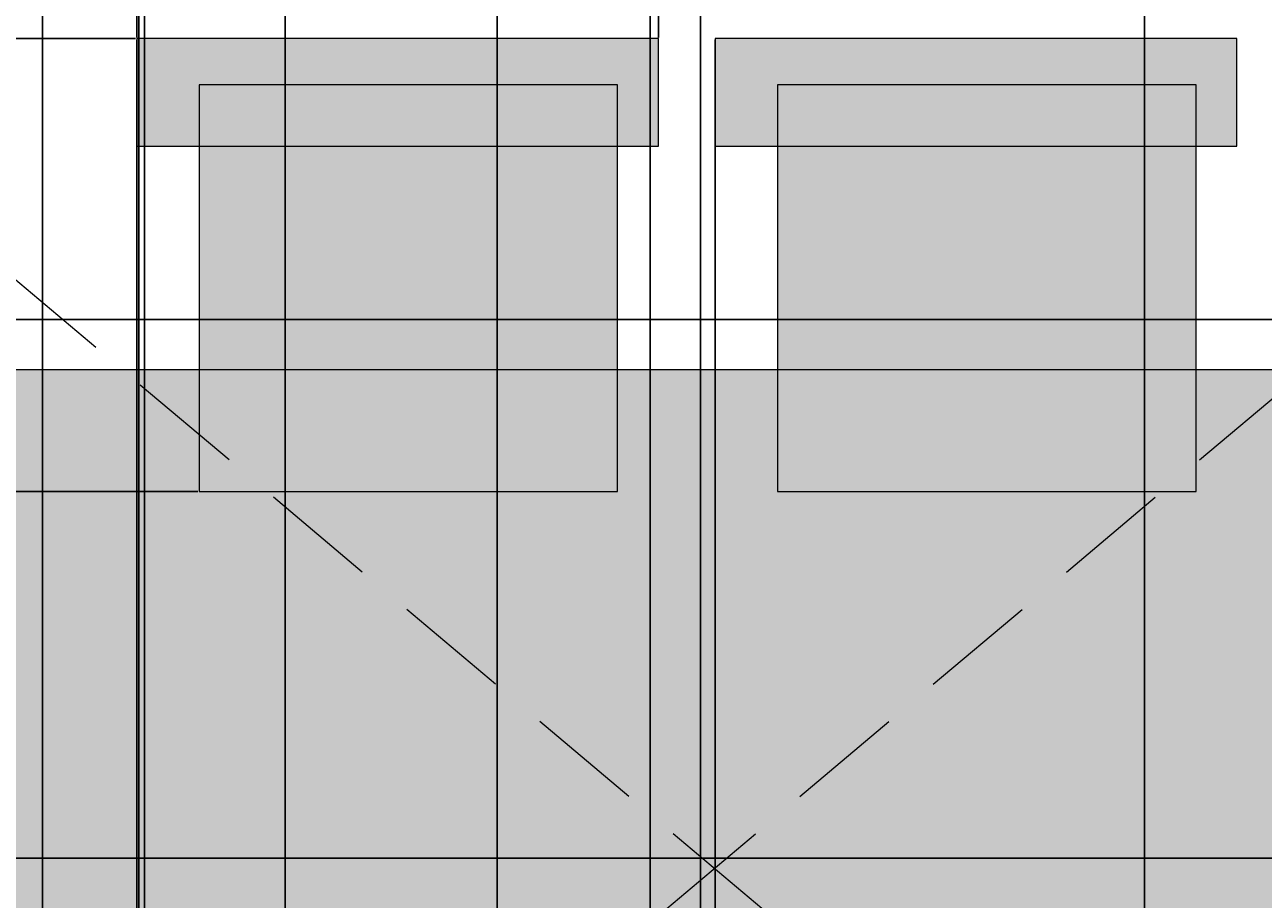
# Model space of a CAD drawing. Units: inches. Extents: x 818 to 1898, y 976 to 2364.
# Tile 73 of 96: x 1305 to 1372, y 1980 to 2027. Entities that reach past the tile are written whole.
import ezdxf

# ---------------------------------------------------------------- set-up
doc = ezdxf.new("R2010")
doc.units = ezdxf.units.IN
doc.header["$LTSCALE"] = 5
doc.header["$MEASUREMENT"] = 0
doc.linetypes.add('HIDDEN', pattern=[0.375, 0.25, -0.125])
for name, color, linetype, lineweight in [('A-ANNO-DIMS', 2, 'Continuous', 18), ('A-FLOR-OVHD', 8, 'HIDDEN', 13), ('A-FURN', 8, 'Continuous', 18), ('A-FURN-PATT', 8, 'Continuous', 9)]:
    doc.layers.add(name, color=color, linetype=linetype, lineweight=lineweight)
doc.styles.get("Standard").update_dxf_attribs({"font": 'arial.ttf'})
doc.dimstyles.get("Standard").update_dxf_attribs({"dimtxt": 0.18, "dimasz": 0.18, "dimexe": 0.18, "dimexo": 0.0625, "dimgap": 0.09, "dimtad": 0, "dimtih": 1, "dimtoh": 1, "dimdec": 4, "dimzin": 0, "dimdsep": 46, "dimtxsty": 'Standard', "dimcen": 0.09, "dimadec": 0, "dimazin": 0, "dimtfac": 1, "dimtdec": 4, "dimtofl": 0, "dimtmove": 0, "dimatfit": 3, "dimfxl": 1, "dimtolj": 1, "dimtzin": 0, "dimarcsym": 0})

# ---------------------------------------------------------------- blocks, each defined once
blk = doc.blocks.new('*D61')
at = {"layer": 'A-ANNO-DIMS', "color": 0, "lineweight": -2, "ltscale": 5, "transparency": 16777216}
for p, q in [((1071.725, 1203.027), (1071.725, 2363.873)), ((1071.905, 2363.693), (1250.936, 2363.693)), ((1430.545, 2363.693), (1251.514, 2363.693)), ((1430.725, 1203.027), (1430.725, 2363.873))]:
    blk.add_line(p, q, dxfattribs=at)
at = {"layer": 'A-ANNO-DIMS', "color": 0, "ltscale": 5, "transparency": 16777216}
for points in [[(1071.905, 2363.723), (1071.905, 2363.663), (1071.725, 2363.693)], [(1430.545, 2363.723), (1430.545, 2363.663), (1430.725, 2363.693)]]:
    blk.add_solid(points, dxfattribs=at)
at = {"layer": 'Defpoints', "color": 0, "ltscale": 5, "transparency": 16777216}
for p in [(1430.725, 2363.693), (1071.725, 1202.964), (1430.725, 1202.964)]:
    blk.add_point(p, dxfattribs=at)
at = {"layer": 'A-ANNO-DIMS', "color": 0, "ltscale": 5, "transparency": 16777216, "insert": (1251.225, 2363.693), "char_height": 0.18, "attachment_point": 5}
blk.add_mtext('\\A1;359', dxfattribs=at)
blk = doc.blocks.new('*D64')
at = {"layer": 'A-ANNO-DIMS', "color": 0, "lineweight": -2, "ltscale": 5, "transparency": 16777216}
for p, q in [((1197.725, 1501.141), (1197.725, 2363.873)), ((1197.905, 2363.693), (1313.935, 2363.693)), ((1430.545, 2363.693), (1314.516, 2363.693)), ((1430.725, 1501.141), (1430.725, 2363.873))]:
    blk.add_line(p, q, dxfattribs=at)
at = {"layer": 'A-ANNO-DIMS', "color": 0, "ltscale": 5, "transparency": 16777216}
for points in [[(1197.905, 2363.723), (1197.905, 2363.663), (1197.725, 2363.693)], [(1430.545, 2363.723), (1430.545, 2363.663), (1430.725, 2363.693)]]:
    blk.add_solid(points, dxfattribs=at)
at = {"layer": 'Defpoints', "color": 0, "ltscale": 5, "transparency": 16777216}
for p in [(1430.725, 2363.693), (1197.725, 1501.078), (1430.725, 1501.078)]:
    blk.add_point(p, dxfattribs=at)
at = {"layer": 'A-ANNO-DIMS', "color": 0, "ltscale": 5, "transparency": 16777216, "insert": (1314.225, 2363.693), "char_height": 0.18, "attachment_point": 5}
blk.add_mtext('\\A1;233', dxfattribs=at)
blk = doc.blocks.new('*D73')
at = {"layer": 'A-ANNO-DIMS', "color": 0, "lineweight": -2, "ltscale": 5, "transparency": 16777216}
for p, q in [((1590.663, 2011.078), (818.026, 2011.078)), ((818.206, 2010.898), (818.206, 1996.76)), ((818.206, 1982.258), (818.206, 1996.396)), ((1590.663, 1982.078), (818.026, 1982.078))]:
    blk.add_line(p, q, dxfattribs=at)
at = {"layer": 'A-ANNO-DIMS', "color": 0, "ltscale": 5, "transparency": 16777216}
for points in [[(818.176, 2010.898), (818.236, 2010.898), (818.206, 2011.078)], [(818.176, 1982.258), (818.236, 1982.258), (818.206, 1982.078)]]:
    blk.add_solid(points, dxfattribs=at)
at = {"layer": 'Defpoints', "color": 0, "ltscale": 5, "transparency": 16777216}
for p in [(818.206, 2011.078), (1590.725, 2011.078), (1590.725, 1982.078)]:
    blk.add_point(p, dxfattribs=at)
at = {"layer": 'A-ANNO-DIMS', "color": 0, "ltscale": 5, "transparency": 16777216, "insert": (818.206, 1996.578), "char_height": 0.18, "attachment_point": 5}
blk.add_mtext('\\A1;29', dxfattribs=at)
blk = doc.blocks.new('*D85')
at = {"layer": 'A-ANNO-DIMS', "color": 0, "lineweight": -2, "ltscale": 5, "transparency": 16777216}
for p, q in [((1258.788, 2053.078), (1897.916, 2053.078)), ((1897.736, 2052.898), (1897.736, 1876.76)), ((1897.736, 1700.258), (1897.736, 1876.396)), ((1258.788, 1700.078), (1897.916, 1700.078))]:
    blk.add_line(p, q, dxfattribs=at)
at = {"layer": 'A-ANNO-DIMS', "color": 0, "ltscale": 5, "transparency": 16777216}
for points in [[(1897.706, 2052.898), (1897.766, 2052.898), (1897.736, 2053.078)], [(1897.706, 1700.258), (1897.766, 1700.258), (1897.736, 1700.078)]]:
    blk.add_solid(points, dxfattribs=at)
at = {"layer": 'Defpoints', "color": 0, "ltscale": 5, "transparency": 16777216}
for p in [(1258.725, 2053.078), (1897.736, 2053.078), (1258.725, 1700.078)]:
    blk.add_point(p, dxfattribs=at)
at = {"layer": 'A-ANNO-DIMS', "color": 0, "ltscale": 5, "transparency": 16777216, "insert": (1897.736, 1876.578), "char_height": 0.18, "attachment_point": 5}
blk.add_mtext('\\A1;353', dxfattribs=at)
blk = doc.blocks.new('*D97')
at = {"layer": 'A-ANNO-DIMS', "color": 0, "lineweight": -2, "ltscale": 5, "transparency": 16777216}
for p, q in [((1284.17, 1071.118), (1284.17, 2363.873)), ((1284.35, 2363.693), (1310.962, 2363.693)), ((1338.361, 2363.693), (1311.749, 2363.693)), ((1338.541, 1071.118), (1338.541, 2363.873))]:
    blk.add_line(p, q, dxfattribs=at)
at = {"layer": 'A-ANNO-DIMS', "color": 0, "ltscale": 5, "transparency": 16777216}
for points in [[(1284.35, 2363.723), (1284.35, 2363.663), (1284.17, 2363.693)], [(1338.361, 2363.723), (1338.361, 2363.663), (1338.541, 2363.693)]]:
    blk.add_solid(points, dxfattribs=at)
at = {"layer": 'Defpoints', "color": 0, "ltscale": 5, "transparency": 16777216}
for p in [(1338.541, 2363.693), (1284.17, 1071.055), (1338.541, 1071.055)]:
    blk.add_point(p, dxfattribs=at)
at = {"layer": 'A-ANNO-DIMS', "color": 0, "ltscale": 5, "transparency": 16777216, "insert": (1311.355, 2363.693), "char_height": 0.18, "attachment_point": 5}
blk.add_mtext('\\A1;54.37', dxfattribs=at)
blk = doc.blocks.new('*D98')
at = {"layer": 'A-ANNO-DIMS', "color": 0, "lineweight": -2, "ltscale": 5, "transparency": 16777216}
for p, q in [((1338.541, 1071.118), (1338.541, 2363.873)), ((1338.721, 2363.693), (1364.815, 2363.693)), ((1391.696, 2363.693), (1365.602, 2363.693)), ((1391.876, 1071.118), (1391.876, 2363.873))]:
    blk.add_line(p, q, dxfattribs=at)
at = {"layer": 'A-ANNO-DIMS', "color": 0, "ltscale": 5, "transparency": 16777216}
for points in [[(1338.721, 2363.723), (1338.721, 2363.663), (1338.541, 2363.693)], [(1391.696, 2363.723), (1391.696, 2363.663), (1391.876, 2363.693)]]:
    blk.add_solid(points, dxfattribs=at)
at = {"layer": 'Defpoints', "color": 0, "ltscale": 5, "transparency": 16777216}
for p in [(1391.876, 2363.693), (1338.541, 1071.055), (1391.876, 1071.055)]:
    blk.add_point(p, dxfattribs=at)
at = {"layer": 'A-ANNO-DIMS', "color": 0, "ltscale": 5, "transparency": 16777216, "insert": (1365.208, 2363.693), "char_height": 0.18, "attachment_point": 5}
blk.add_mtext('\\A1;53.33', dxfattribs=at)
blk = doc.blocks.new('*D165')
at = {"layer": 'A-ANNO-DIMS', "color": 0, "lineweight": -2, "ltscale": 5, "transparency": 16777216}
for p, q in [((1283.818, 1510.141), (1283.818, 2363.873)), ((1283.998, 2363.693), (1324.088, 2363.693)), ((1364.966, 2363.693), (1324.876, 2363.693)), ((1365.146, 1510.141), (1365.146, 2363.873))]:
    blk.add_line(p, q, dxfattribs=at)
at = {"layer": 'A-ANNO-DIMS', "color": 0, "ltscale": 5, "transparency": 16777216}
for points in [[(1283.998, 2363.723), (1283.998, 2363.663), (1283.818, 2363.693)], [(1364.966, 2363.723), (1364.966, 2363.663), (1365.146, 2363.693)]]:
    blk.add_solid(points, dxfattribs=at)
at = {"layer": 'Defpoints', "color": 0, "ltscale": 5, "transparency": 16777216}
for p in [(1365.146, 2363.693), (1283.818, 1510.078), (1365.146, 1510.078)]:
    blk.add_point(p, dxfattribs=at)
at = {"layer": 'A-ANNO-DIMS', "color": 0, "ltscale": 5, "transparency": 16777216, "insert": (1324.482, 2363.693), "char_height": 0.18, "attachment_point": 5}
blk.add_mtext('\\A1;81.33', dxfattribs=at)
blk = doc.blocks.new('*D207')
at = {"layer": 'A-ANNO-DIMS', "color": 0, "lineweight": -2, "ltscale": 5, "transparency": 16777216}
for p, q in [((1590.663, 2044.078), (818.026, 2044.078)), ((818.206, 2043.898), (818.206, 2027.76)), ((818.206, 2011.258), (818.206, 2027.396)), ((1590.663, 2011.078), (818.026, 2011.078))]:
    blk.add_line(p, q, dxfattribs=at)
at = {"layer": 'A-ANNO-DIMS', "color": 0, "ltscale": 5, "transparency": 16777216}
for points in [[(818.176, 2043.898), (818.236, 2043.898), (818.206, 2044.078)], [(818.176, 2011.258), (818.236, 2011.258), (818.206, 2011.078)]]:
    blk.add_solid(points, dxfattribs=at)
at = {"layer": 'Defpoints', "color": 0, "ltscale": 5, "transparency": 16777216}
for p in [(818.206, 2044.078), (1590.725, 2044.078), (1590.725, 2011.078)]:
    blk.add_point(p, dxfattribs=at)
at = {"layer": 'A-ANNO-DIMS', "color": 0, "ltscale": 5, "transparency": 16777216, "insert": (818.206, 2027.578), "char_height": 0.18, "attachment_point": 5}
blk.add_mtext('\\A1;33', dxfattribs=at)
blk = doc.blocks.new('*D235')
at = {"layer": 'A-ANNO-DIMS', "color": 0, "lineweight": -2, "ltscale": 5, "transparency": 16777216}
for p, q in [((1310.908, 2026.27), (1310.908, 2363.873)), ((1311.088, 2363.693), (1324.485, 2363.693)), ((1338.812, 2363.693), (1325.414, 2363.693)), ((1338.992, 2026.27), (1338.992, 2363.873))]:
    blk.add_line(p, q, dxfattribs=at)
at = {"layer": 'A-ANNO-DIMS', "color": 0, "ltscale": 5, "transparency": 16777216}
for points in [[(1311.088, 2363.723), (1311.088, 2363.663), (1310.908, 2363.693)], [(1338.812, 2363.723), (1338.812, 2363.663), (1338.992, 2363.693)]]:
    blk.add_solid(points, dxfattribs=at)
at = {"layer": 'Defpoints', "color": 0, "ltscale": 5, "transparency": 16777216}
for p in [(1338.992, 2363.693), (1310.908, 2026.207), (1338.992, 2026.207)]:
    blk.add_point(p, dxfattribs=at)
at = {"layer": 'A-ANNO-DIMS', "color": 0, "ltscale": 5, "transparency": 16777216, "insert": (1324.95, 2363.693), "char_height": 0.18, "attachment_point": 5}
blk.add_mtext('\\A1;28.084', dxfattribs=at)
blk = doc.blocks.new('*D236')
at = {"layer": 'A-ANNO-DIMS', "color": 0, "lineweight": -2, "ltscale": 5, "transparency": 16777216}
for p, q in [((1310.908, 2026.145), (1310.908, 975.663)), ((1342.045, 2026.145), (1342.045, 975.663)), ((1311.088, 975.843), (1326.083, 975.843)), ((1341.865, 975.843), (1326.87, 975.843))]:
    blk.add_line(p, q, dxfattribs=at)
at = {"layer": 'A-ANNO-DIMS', "color": 0, "ltscale": 5, "transparency": 16777216}
for points in [[(1311.088, 975.873), (1311.088, 975.813), (1310.908, 975.843)], [(1341.865, 975.873), (1341.865, 975.813), (1342.045, 975.843)]]:
    blk.add_solid(points, dxfattribs=at)
at = {"layer": 'Defpoints', "color": 0, "ltscale": 5, "transparency": 16777216}
for p in [(1310.908, 2026.207), (1342.045, 2026.207), (1342.045, 975.843)]:
    blk.add_point(p, dxfattribs=at)
at = {"layer": 'A-ANNO-DIMS', "color": 0, "ltscale": 5, "transparency": 16777216, "insert": (1326.476, 975.843), "char_height": 0.18, "attachment_point": 5}
blk.add_mtext('\\A1;31.14', dxfattribs=at)
blk = doc.blocks.new('*D237')
at = {"layer": 'A-ANNO-DIMS', "color": 0, "lineweight": -2, "ltscale": 5, "transparency": 16777216}
for p, q in [((1310.845, 2026.207), (818.026, 2026.207)), ((818.206, 2026.027), (818.206, 2014.198)), ((818.206, 2002.005), (818.206, 2013.834)), ((1314.197, 2001.825), (818.026, 2001.825))]:
    blk.add_line(p, q, dxfattribs=at)
at = {"layer": 'A-ANNO-DIMS', "color": 0, "ltscale": 5, "transparency": 16777216}
for points in [[(818.176, 2026.027), (818.236, 2026.027), (818.206, 2026.207)], [(818.176, 2002.005), (818.236, 2002.005), (818.206, 2001.825)]]:
    blk.add_solid(points, dxfattribs=at)
at = {"layer": 'Defpoints', "color": 0, "ltscale": 5, "transparency": 16777216}
for p in [(1310.908, 2026.207), (818.206, 2001.825), (1314.26, 2001.825)]:
    blk.add_point(p, dxfattribs=at)
at = {"layer": 'A-ANNO-DIMS', "color": 0, "ltscale": 5, "transparency": 16777216, "insert": (818.206, 2014.016), "char_height": 0.18, "attachment_point": 5}
blk.add_mtext('\\A1;24.383', dxfattribs=at)
blk = doc.blocks.new('*D252')
at = {"layer": 'A-ANNO-DIMS', "color": 0, "lineweight": -2, "ltscale": 5, "transparency": 16777216}
for p, q in [((1330.305, 2053.016), (1330.305, 975.663)), ((1388.031, 2053.016), (1388.031, 975.663)), ((1330.485, 975.843), (1358.775, 975.843)), ((1387.851, 975.843), (1359.562, 975.843))]:
    blk.add_line(p, q, dxfattribs=at)
at = {"layer": 'A-ANNO-DIMS', "color": 0, "ltscale": 5, "transparency": 16777216}
for points in [[(1330.485, 975.873), (1330.485, 975.813), (1330.305, 975.843)], [(1387.851, 975.873), (1387.851, 975.813), (1388.031, 975.843)]]:
    blk.add_solid(points, dxfattribs=at)
at = {"layer": 'Defpoints', "color": 0, "ltscale": 5, "transparency": 16777216}
for p in [(1330.305, 2053.078), (1388.031, 2053.078), (1388.031, 975.843)]:
    blk.add_point(p, dxfattribs=at)
at = {"layer": 'A-ANNO-DIMS', "color": 0, "ltscale": 5, "transparency": 16777216, "insert": (1359.168, 975.843), "char_height": 0.18, "attachment_point": 5}
blk.add_mtext('\\A1;57.73', dxfattribs=at)
blk = doc.blocks.new('*D254')
at = {"layer": 'A-ANNO-DIMS', "color": 0, "lineweight": -2, "ltscale": 5, "transparency": 16777216}
for p, q in [((1267.725, 2044.016), (1267.725, 975.663)), ((1330.305, 2044.016), (1330.305, 975.663)), ((1267.905, 975.843), (1298.621, 975.843)), ((1330.125, 975.843), (1299.409, 975.843))]:
    blk.add_line(p, q, dxfattribs=at)
at = {"layer": 'A-ANNO-DIMS', "color": 0, "ltscale": 5, "transparency": 16777216}
for points in [[(1267.905, 975.873), (1267.905, 975.813), (1267.725, 975.843)], [(1330.125, 975.873), (1330.125, 975.813), (1330.305, 975.843)]]:
    blk.add_solid(points, dxfattribs=at)
at = {"layer": 'Defpoints', "color": 0, "ltscale": 5, "transparency": 16777216}
for p in [(1267.725, 2044.078), (1330.305, 2044.078), (1330.305, 975.843)]:
    blk.add_point(p, dxfattribs=at)
at = {"layer": 'A-ANNO-DIMS', "color": 0, "ltscale": 5, "transparency": 16777216, "insert": (1299.015, 975.843), "char_height": 0.18, "attachment_point": 5}
blk.add_mtext('\\A1;62.58', dxfattribs=at)
blk = doc.blocks.new('*D269')
at = {"layer": 'A-ANNO-DIMS', "color": 0, "lineweight": -2, "ltscale": 5, "transparency": 16777216}
for p, q in [((1246.938, 1534.141), (1246.938, 2363.873)), ((1247.118, 2363.693), (1293.706, 2363.693)), ((1341.079, 2363.693), (1294.491, 2363.693)), ((1341.259, 1534.141), (1341.259, 2363.873))]:
    blk.add_line(p, q, dxfattribs=at)
at = {"layer": 'A-ANNO-DIMS', "color": 0, "ltscale": 5, "transparency": 16777216}
for points in [[(1247.118, 2363.723), (1247.118, 2363.663), (1246.938, 2363.693)], [(1341.079, 2363.723), (1341.079, 2363.663), (1341.259, 2363.693)]]:
    blk.add_solid(points, dxfattribs=at)
at = {"layer": 'Defpoints', "color": 0, "ltscale": 5, "transparency": 16777216}
for p in [(1341.259, 2363.693), (1246.938, 1534.078), (1341.259, 1534.078)]:
    blk.add_point(p, dxfattribs=at)
at = {"layer": 'A-ANNO-DIMS', "color": 0, "ltscale": 5, "transparency": 16777216, "insert": (1294.099, 2363.693), "char_height": 0.18, "attachment_point": 5}
blk.add_mtext('\\A1;94.32', dxfattribs=at)
blk = doc.blocks.new('*D274')
at = {"layer": 'A-ANNO-DIMS', "color": 0, "lineweight": -2, "ltscale": 5, "transparency": 16777216}
for p, q in [((1311.025, 1897.929), (1311.025, 2363.873)), ((1311.205, 2363.693), (1344.007, 2363.693)), ((1377.599, 2363.693), (1344.797, 2363.693)), ((1377.779, 1897.929), (1377.779, 2363.873))]:
    blk.add_line(p, q, dxfattribs=at)
at = {"layer": 'A-ANNO-DIMS', "color": 0, "ltscale": 5, "transparency": 16777216}
for points in [[(1311.205, 2363.723), (1311.205, 2363.663), (1311.025, 2363.693)], [(1377.599, 2363.723), (1377.599, 2363.663), (1377.779, 2363.693)]]:
    blk.add_solid(points, dxfattribs=at)
at = {"layer": 'Defpoints', "color": 0, "ltscale": 5, "transparency": 16777216}
for p in [(1377.779, 2363.693), (1311.025, 1897.866), (1377.779, 1897.866)]:
    blk.add_point(p, dxfattribs=at)
at = {"layer": 'A-ANNO-DIMS', "color": 0, "ltscale": 5, "transparency": 16777216, "insert": (1344.402, 2363.693), "char_height": 0.18, "attachment_point": 5}
blk.add_mtext('\\A1;66.75', dxfattribs=at)
blk = doc.blocks.new('*D281')
at = {"layer": 'A-ANNO-DIMS', "color": 0, "lineweight": -2, "ltscale": 5, "transparency": 16777216}
for p, q in [((1250.303, 1913.703), (1250.303, 2363.873)), ((1250.483, 2363.693), (1420.121, 2363.693)), ((1590.545, 2363.693), (1420.907, 2363.693)), ((1590.725, 2011.141), (1590.725, 2363.873))]:
    blk.add_line(p, q, dxfattribs=at)
at = {"layer": 'A-ANNO-DIMS', "color": 0, "ltscale": 5, "transparency": 16777216}
for points in [[(1250.483, 2363.723), (1250.483, 2363.663), (1250.303, 2363.693)], [(1590.545, 2363.723), (1590.545, 2363.663), (1590.725, 2363.693)]]:
    blk.add_solid(points, dxfattribs=at)
at = {"layer": 'Defpoints', "color": 0, "ltscale": 5, "transparency": 16777216}
for p in [(1590.725, 2363.693), (1590.725, 2011.078), (1250.303, 1913.64)]:
    blk.add_point(p, dxfattribs=at)
at = {"layer": 'A-ANNO-DIMS', "color": 0, "ltscale": 5, "transparency": 16777216, "insert": (1420.514, 2363.693), "char_height": 0.18, "attachment_point": 5}
blk.add_mtext('\\A1;340.4', dxfattribs=at)
blk = doc.blocks.new('*D286')
at = {"layer": 'A-ANNO-DIMS', "color": 0, "lineweight": -2, "ltscale": 5, "transparency": 16777216}
for p, q in [((1305.828, 1851.971), (1305.828, 2363.873)), ((1306.008, 2363.693), (1308.184, 2363.693)), ((1311.147, 2363.693), (1308.971, 2363.693)), ((1311.327, 1853.812), (1311.327, 2363.873))]:
    blk.add_line(p, q, dxfattribs=at)
at = {"layer": 'A-ANNO-DIMS', "color": 0, "ltscale": 5, "transparency": 16777216}
for points in [[(1306.008, 2363.723), (1306.008, 2363.663), (1305.828, 2363.693)], [(1311.147, 2363.723), (1311.147, 2363.663), (1311.327, 2363.693)]]:
    blk.add_solid(points, dxfattribs=at)
at = {"layer": 'Defpoints', "color": 0, "ltscale": 5, "transparency": 16777216}
for p in [(1305.828, 2363.693), (1311.327, 1853.75), (1305.828, 1851.908)]:
    blk.add_point(p, dxfattribs=at)
at = {"layer": 'A-ANNO-DIMS', "color": 0, "ltscale": 5, "transparency": 16777216, "insert": (1308.577, 2363.693), "char_height": 0.18, "attachment_point": 5}
blk.add_mtext('\\A1;5.499', dxfattribs=at)
blk = doc.blocks.new('*D290')
at = {"layer": 'A-ANNO-DIMS', "color": 0, "lineweight": -2, "ltscale": 5, "transparency": 16777216}
for p, q in [((1302.983, 1599.435), (1302.983, 2363.873)), ((1303.163, 2363.693), (1310.57, 2363.693)), ((1318.713, 2363.693), (1311.306, 2363.693)), ((1318.893, 1607.833), (1318.893, 2363.873))]:
    blk.add_line(p, q, dxfattribs=at)
at = {"layer": 'A-ANNO-DIMS', "color": 0, "ltscale": 5, "transparency": 16777216}
for points in [[(1303.163, 2363.723), (1303.163, 2363.663), (1302.983, 2363.693)], [(1318.713, 2363.723), (1318.713, 2363.663), (1318.893, 2363.693)]]:
    blk.add_solid(points, dxfattribs=at)
at = {"layer": 'Defpoints', "color": 0, "ltscale": 5, "transparency": 16777216}
for p in [(1318.893, 2363.693), (1318.893, 1607.771), (1302.983, 1599.372)]:
    blk.add_point(p, dxfattribs=at)
at = {"layer": 'A-ANNO-DIMS', "color": 0, "ltscale": 5, "transparency": 16777216, "insert": (1310.938, 2363.693), "char_height": 0.18, "attachment_point": 5}
blk.add_mtext('\\A1;15.91', dxfattribs=at)

msp = doc.modelspace()

# ---------------------------------------------------------------- hatches: boundary and pattern name
at = {"layer": 'A-FURN-PATT', "ltscale": 5}
h = msp.add_hatch(color=256, dxfattribs=at)
h.dxf.hatch_style = 1
h.paths.add_polyline_path([(1341.9997, 1981.5338), (1317.9034, 2001.8247), (1314.2595, 2001.8247), (1314.2595, 2004.893), (1310.1046, 2008.3917), (1303.9314, 2008.3917), (1303.9314, 1953.0408), (1308.1629, 1953.0408), (1314.2595, 1958.1746), (1314.2595, 1959.6079), (1315.9616, 1959.6079)])
h.paths.add_polyline_path([(1341.9997, 1981.5338), (1315.9616, 1959.6079), (1336.7936, 1959.6079), (1336.7936, 1953.0408), (1345.3966, 1953.0408), (1345.3966, 1959.6079), (1368.0379, 1959.6079)])
h.paths.add_polyline_path([(1402.518, 2008.3917), (1398.8475, 2008.3917), (1398.8475, 2001.8247), (1376.3134, 2001.8247), (1376.3134, 2008.3917), (1373.8948, 2008.3917), (1367.9307, 2003.3695), (1367.9307, 2001.8247), (1366.0961, 2001.8247), (1341.9997, 1981.5338), (1368.0379, 1959.6079), (1375.8366, 1953.0408), (1376.3134, 1953.0408), (1376.3134, 1959.6079), (1398.8475, 1959.6079), (1398.8475, 1953.0408), (1402.518, 1953.0408)])
h.paths.add_polyline_path([(1366.0961, 2001.8247), (1345.3966, 2001.8247), (1345.3966, 2008.3917), (1336.7936, 2008.3917), (1336.7936, 2001.8247), (1317.9034, 2001.8247), (1341.9997, 1981.5338)])
h.paths.add_polyline_path([(1336.7936, 1959.6079), (1315.9616, 1959.6079), (1314.2595, 1958.1746), (1314.2595, 1953.0408), (1336.7936, 1953.0408)], flags=17)
h.paths.add_polyline_path([(1367.9307, 1959.6079), (1345.3966, 1959.6079), (1345.3966, 1953.0408), (1367.9307, 1953.0408)], flags=17)
h.paths.add_polyline_path([(1398.8475, 1959.6079), (1376.3134, 1959.6079), (1376.3134, 1953.0408), (1398.8475, 1953.0408)], flags=17)
h.paths.add_polyline_path([(1368.0379, 1959.6079), (1367.9307, 1959.6079), (1367.9307, 1953.0408), (1375.8366, 1953.0408)], flags=17)
h.paths.add_polyline_path([(1314.2595, 1958.1746), (1308.1629, 1953.0408), (1314.2595, 1953.0408)], flags=17)
h.paths.add_polyline_path([(1315.9616, 1959.6079), (1314.2595, 1959.6079), (1314.2595, 1958.1746)], flags=16)
h.paths.add_polyline_path([(1314.2595, 2008.3917), (1310.1046, 2008.3917), (1314.2595, 2004.893)], flags=17)
h.paths.add_polyline_path([(1336.7936, 2008.3917), (1314.2595, 2008.3917), (1314.2595, 2004.893), (1317.9034, 2001.8247), (1336.7936, 2001.8247)], flags=17)
h.paths.add_polyline_path([(1314.2595, 2004.893), (1314.2595, 2001.8247), (1317.9034, 2001.8247)], flags=16)
h.paths.add_polyline_path([(1367.9307, 2008.3917), (1345.3966, 2008.3917), (1345.3966, 2001.8247), (1366.0961, 2001.8247), (1367.9307, 2003.3695)], flags=17)
h.paths.add_polyline_path([(1398.8475, 2008.3917), (1376.3134, 2008.3917), (1376.3134, 2001.8247), (1398.8475, 2001.8247)], flags=17)
h.paths.add_polyline_path([(1373.8948, 2008.3917), (1367.9307, 2008.3917), (1367.9307, 2003.3695)], flags=17)
h.paths.add_polyline_path([(1367.9307, 2003.3695), (1366.0961, 2001.8247), (1367.9307, 2001.8247)], flags=16)
h.paths.add_polyline_path([(1546.1595, 2044.0782), (1451.7698, 2044.0782), (1451.7698, 2020.0782), (1546.1595, 2020.0782)])
h.paths.add_polyline_path([(1492.0729, 2040.001, 0.431429), (1491.8238, 2040.251), (1491.3087, 2040.251, 0.415217), (1491.0729, 2040.001)], flags=16)
h.paths.add_polyline_path([(1481.8346, 2039.6036), (1511.886, 2039.6036), (1511.886, 2024.9917), (1481.8346, 2024.9917)], flags=16)
h.paths.add_polyline_path([(1491.0729, 2039.4857), (1491.0729, 2039.501), (1492.0729, 2039.501, -0.4117484), (1491.8401, 2039.251), (1491.8229, 2039.251), (1491.8229, 2039.2509, 0.4325918), (1492.0729, 2039.501), (1491.0729, 2039.501, 0.432604), (1491.3229, 2039.2509), (1491.3229, 2039.251), (1491.325, 2039.251, -0.4165823)], flags=0)
h.paths.add_polyline_path([(1485.3701, 2030.9622), (1485.3701, 2034.3556, -0.4142136), (1488.3701, 2037.3556), (1490.3421, 2037.3556, -0.0779193), (1491.0729, 2038.751), (1495.0729, 2038.751, -0.3148679), (1496.07, 2037.1201, -0.3016609), (1497.9049, 2034.3556), (1497.9049, 2030.9622, -0.4142136), (1494.9049, 2027.9622), (1488.3701, 2027.9622, -0.4142136)], flags=0)
h.paths.add_polyline_path([(1490.3229, 2035.751, 0.2655648), (1491.3229, 2036.751), (1491.3229, 2037.126), (1491.0729, 2037.126, -0.7914183), (1490.5434, 2037.251, -0.7914183), (1491.0729, 2037.376), (1491.3229, 2037.376), (1491.3229, 2037.751), (1492.0729, 2037.751), (1492.0729, 2037.376), (1492.3229, 2037.376, -0.7914183), (1492.8524, 2037.251, -0.7914183), (1492.3229, 2037.126), (1492.1491, 2037.126, -0.0866263), (1492.5376, 2036.0294, 0.1070481), (1493.0729, 2035.751), (1490.3229, 2035.751)], flags=0)
h.paths.add_polyline_path([(1491.9774, 2037.251, -1), (1491.4184, 2037.251, -1)], flags=0)
h.paths.add_polyline_path([(1500.0743, 2028.6045), (1500.0743, 2029.4074), (1510.8414, 2029.4074), (1510.8414, 2028.6045)], flags=0)
h.paths.add_polyline_path([(1500.0743, 2030.5314), (1500.0743, 2031.3342), (1510.8414, 2031.3342), (1510.8414, 2030.5314)], flags=0)
h.paths.add_polyline_path([(1500.0743, 2032.94), (1500.0743, 2033.7428), (1510.8414, 2033.7428), (1510.8414, 2032.94)], flags=0)
h.paths.add_polyline_path([(1500.0743, 2035.7499), (1500.0743, 2036.5528), (1510.8414, 2036.5528), (1510.8414, 2035.7499)], flags=0)
h.paths.add_polyline_path([(1590.7251, 2044.0782), (1576.1595, 2044.0782), (1576.1595, 2020.0782), (1590.7251, 2020.0782)])
h.paths.add_polyline_path([(1668.4429, 2044.0782), (1599.7252, 2044.0782), (1599.7252, 2020.0782), (1668.4429, 2020.0782)])
h.paths.add_polyline_path([(1621.2588, 2040.001, 0.431429), (1621.0097, 2040.251), (1620.4946, 2040.251, 0.415217), (1620.2588, 2040.001)], flags=16)
h.paths.add_polyline_path([(1611.0205, 2024.9917), (1611.0205, 2039.6036), (1641.0719, 2039.6036), (1641.0719, 2024.9917)], flags=16)
h.paths.add_polyline_path([(1620.2588, 2039.4857), (1620.2588, 2039.501), (1621.2588, 2039.501, -0.4117484), (1621.026, 2039.251), (1621.0088, 2039.251), (1621.0088, 2039.2509, 0.4325918), (1621.2588, 2039.501), (1620.2588, 2039.501, 0.432604), (1620.5088, 2039.2509), (1620.5088, 2039.251), (1620.5109, 2039.251, -0.4165823)], flags=0)
h.paths.add_polyline_path([(1614.556, 2030.9622), (1614.556, 2034.3556, -0.4142136), (1617.556, 2037.3556), (1619.528, 2037.3556, -0.0779193), (1620.2588, 2038.751), (1624.2588, 2038.751, -0.3148679), (1625.2559, 2037.1201, -0.3016609), (1627.0908, 2034.3556), (1627.0908, 2030.9622, -0.4142136), (1624.0908, 2027.9622), (1617.556, 2027.9622, -0.4142136)], flags=0)
h.paths.add_polyline_path([(1619.5088, 2035.751, 0.2655648), (1620.5088, 2036.751), (1620.5088, 2037.126), (1620.2588, 2037.126, -0.7914183), (1619.7293, 2037.251, -0.7914183), (1620.2588, 2037.376), (1620.5088, 2037.376), (1620.5088, 2037.751), (1621.2588, 2037.751), (1621.2588, 2037.376), (1621.5088, 2037.376, -0.7914183), (1622.0383, 2037.251, -0.7914183), (1621.5088, 2037.126), (1621.335, 2037.126, -0.0866263), (1621.7235, 2036.0294, 0.1070481), (1622.2588, 2035.751), (1619.5088, 2035.751)], flags=0)
h.paths.add_polyline_path([(1620.6043, 2037.251, -1), (1621.1633, 2037.251, -1)], flags=0)
h.paths.add_polyline_path([(1629.2602, 2028.6045), (1629.2602, 2029.4074), (1640.0273, 2029.4074), (1640.0273, 2028.6045)], flags=0)
h.paths.add_polyline_path([(1629.2602, 2030.5314), (1629.2602, 2031.3342), (1640.0273, 2031.3342), (1640.0273, 2030.5314)], flags=0)
h.paths.add_polyline_path([(1629.2602, 2032.94), (1629.2602, 2033.7428), (1640.0273, 2033.7428), (1640.0273, 2032.94)], flags=0)
h.paths.add_polyline_path([(1629.2602, 2035.7499), (1629.2602, 2036.5528), (1640.0273, 2036.5528), (1640.0273, 2035.7499)], flags=0)
h.paths.add_polyline_path([(1705.7252, 2044.0782), (1698.4429, 2044.0782), (1698.4429, 2020.0782), (1705.7252, 2020.0782)])
h.paths.add_polyline_path([(1705.7252, 1972.0782), (1599.7252, 1972.0782), (1599.7252, 1948.0782), (1705.7252, 1948.0782)])
h.paths.add_polyline_path([(1550.0109, 1979.2444), (1483.5451, 1979.2444), (1483.5451, 1948.6602), (1550.0109, 1948.6602)])
h.paths.add_polyline_path([(1490.2586, 1948.6602), (1488.2586, 1948.6602), (1488.2586, 1941.1742, 0.4142136), (1491.2586, 1938.1742), (1500.7446, 1938.1742, -0.4142136)])
h.paths.add_polyline_path([(1513.2306, 1941.1742), (1513.2306, 1948.6602), (1511.2306, 1948.6602, -0.4142136), (1500.7446, 1938.1742), (1510.2306, 1938.1742, 0.4142136)])
h.paths.add_polyline_path([(1518.778, 1948.6602), (1516.778, 1948.6602), (1516.778, 1941.1742, 0.4142136), (1519.778, 1938.1742), (1529.264, 1938.1742, -0.4142136)])
h.paths.add_polyline_path([(1541.75, 1941.1742), (1541.75, 1948.6602), (1539.75, 1948.6602, -0.4142136), (1529.264, 1938.1742), (1538.75, 1938.1742, 0.4142136)])
h.paths.add_polyline_path([(1590.7251, 1900.0782), (1519.6413, 1900.0782), (1519.6413, 1876.0782), (1590.7251, 1876.0782)])
h = msp.add_hatch(color=256, dxfattribs=at)
h.dxf.hatch_style = 1
h.paths.add_polyline_path([(1336.7936, 1953.0408), (1314.2595, 1953.0408), (1314.2595, 1941.0096), (1336.7936, 1941.0096)])
h.paths.add_polyline_path([(1338.9915, 1941.0096), (1336.7936, 1941.0096), (1336.7936, 1937.7177), (1314.2595, 1937.7177), (1314.2595, 1941.0096), (1310.9077, 1941.0096), (1310.9077, 1935.2252), (1338.9915, 1935.2252)])
h.paths.add_polyline_path([(1336.7936, 1941.0096), (1314.2595, 1941.0096), (1314.2595, 1937.7177), (1336.7936, 1937.7177)], flags=17)
h.paths.add_polyline_path([(1367.9307, 1959.6079), (1345.3966, 1959.6079), (1345.3966, 1941.0096), (1367.9307, 1941.0096)])
h.paths.add_polyline_path([(1398.8475, 1953.0408), (1376.3134, 1953.0408), (1376.3134, 1952.6393), (1390.1242, 1941.0096), (1398.8475, 1941.0096)])
h.paths.add_polyline_path([(1376.3134, 1952.6393), (1376.3134, 1941.0096), (1390.1242, 1941.0096)], flags=17)
h.paths.add_polyline_path([(1370.1286, 1941.0096), (1367.9307, 1941.0096), (1367.9307, 1937.7177), (1345.3966, 1937.7177), (1345.3966, 1941.0096), (1342.0448, 1941.0096), (1342.0448, 1935.2252), (1370.1286, 1935.2252)])
h.paths.add_polyline_path([(1367.9307, 1941.0096), (1345.3966, 1941.0096), (1345.3966, 1937.7177), (1367.9307, 1937.7177)], flags=17)
h.paths.add_polyline_path([(1390.1242, 1941.0096), (1376.3134, 1941.0096), (1376.3134, 1937.7177), (1394.0336, 1937.7177)], flags=17)
h.paths.add_polyline_path([(1394.0336, 1937.7177), (1376.3134, 1937.7177), (1376.3134, 1941.0096), (1372.9616, 1941.0096), (1372.9616, 1935.2252), (1396.9935, 1935.2252)])
h.paths.add_polyline_path([(1398.8475, 1941.0096), (1390.1242, 1941.0096), (1394.0336, 1937.7177), (1398.8475, 1937.7177)])
h.paths.add_polyline_path([(1401.0455, 1941.0096), (1398.8475, 1941.0096), (1398.8475, 1937.7177), (1394.0336, 1937.7177), (1396.9935, 1935.2252), (1401.0455, 1935.2252)])
h.paths.add_polyline_path([(1336.7936, 2020.4229), (1314.2595, 2020.4229), (1314.2595, 2008.3917), (1336.7936, 2008.3917)])
h.paths.add_polyline_path([(1336.7936, 2023.7149), (1314.2595, 2023.7149), (1314.2595, 2020.4229), (1336.7936, 2020.4229)], flags=17)
h.paths.add_polyline_path([(1338.9915, 2026.2074), (1310.9077, 2026.2074), (1310.9077, 2020.4229), (1314.2595, 2020.4229), (1314.2595, 2023.7149), (1336.7936, 2023.7149), (1336.7936, 2020.4229), (1338.9915, 2020.4229)])
h.paths.add_polyline_path([(1367.9307, 2023.7149), (1345.3966, 2023.7149), (1345.3966, 2020.4229), (1367.9307, 2020.4229)], flags=17)
h.paths.add_polyline_path([(1370.1286, 2026.2074), (1342.0448, 2026.2074), (1342.0448, 2020.4229), (1345.3966, 2020.4229), (1345.3966, 2023.7149), (1367.9307, 2023.7149), (1367.9307, 2020.4229), (1370.1286, 2020.4229)])
h.paths.add_polyline_path([(1367.9307, 2020.4229), (1345.3966, 2020.4229), (1345.3966, 2008.3917), (1367.9307, 2008.3917)])
h.paths.add_polyline_path([(1398.8475, 2020.4229), (1388.1824, 2020.4229), (1376.3134, 2010.4284), (1376.3134, 2008.3917), (1398.8475, 2008.3917)])
h.paths.add_polyline_path([(1392.0918, 2023.7149), (1376.3134, 2023.7149), (1376.3134, 2020.4229), (1388.1824, 2020.4229)], flags=17)
h.paths.add_polyline_path([(1388.1824, 2020.4229), (1376.3134, 2020.4229), (1376.3134, 2010.4284)], flags=17)
h.paths.add_polyline_path([(1395.0518, 2026.2074), (1372.9616, 2026.2074), (1372.9616, 2020.4229), (1376.3134, 2020.4229), (1376.3134, 2023.7149), (1392.0918, 2023.7149)])
h.paths.add_polyline_path([(1398.8475, 2023.7149), (1392.0918, 2023.7149), (1388.1824, 2020.4229), (1398.8475, 2020.4229)])
h.paths.add_polyline_path([(1401.0455, 2026.2074), (1395.0518, 2026.2074), (1392.0918, 2023.7149), (1398.8475, 2023.7149), (1398.8475, 2020.4229), (1401.0455, 2020.4229)])
h.paths.add_polyline_path([(1327.0339, 1897.8663), (1311.025, 1897.8663), (1311.025, 1876.0782), (1327.0339, 1876.0782)])
h.paths.add_polyline_path([(1377.7791, 1897.8663), (1359.9579, 1897.8663), (1359.9579, 1876.0782), (1377.7791, 1876.0782)])
h.paths.add_polyline_path([(1430.7251, 1541.0439), (1406.7252, 1541.0439), (1406.7252, 1525.9965), (1430.7251, 1525.9965)])
h.paths.add_polyline_path([(1430.7251, 1587.4164), (1406.7252, 1587.4164), (1406.7252, 1570.9187), (1430.7251, 1570.9187)])

# ---------------------------------------------------------------- linework, layer by layer
at = {"layer": 'A-FLOR-OVHD', "ltscale": 5}
for p, q in [((1416.2743, 1918.9894), (1267.7251, 2044.0782)), ((1267.7251, 1918.9894), (1416.2743, 2044.0782))]:
    msp.add_line(p, q, dxfattribs=at)
at = {"layer": 'A-FURN'}
for points in [[(1310.9077, 2020.4229), (1338.9915, 2020.4229), (1338.9915, 2026.2074), (1310.9077, 2026.2074)], [(1342.0448, 2020.4229), (1370.1286, 2020.4229), (1370.1286, 2026.2074), (1342.0448, 2026.2074)], [(1314.2595, 2001.8247), (1336.7936, 2001.8247), (1336.7936, 2023.7149), (1314.2595, 2023.7149)], [(1345.3966, 2001.8247), (1367.9307, 2001.8247), (1367.9307, 2023.7149), (1345.3966, 2023.7149)], [(1303.9314, 2008.3917), (1402.518, 2008.3917), (1402.518, 1953.0408), (1303.9314, 1953.0408)]]:
    msp.add_lwpolyline(points, close=True, dxfattribs=at)

# ---------------------------------------------------------------- dimensions: what is measured, and where the dimension line sits
at = {"layer": 'A-ANNO-DIMS', "ltscale": 5}
for base, p1, p2, override, picture, middle in [((1430.7251, 2363.6929), (1071.7251, 1202.9642), (1430.7251, 1202.9642), {"dimdec": 0, "dimlfac": 1, "dimrnd": 0, "dimzin": 0, "dimdsep": 46, "dimlunit": 2}, '*D61', (1251.2251, 2363.6929)), ((1430.7251, 2363.6929), (1197.7251, 1501.0782), (1430.7251, 1501.0782), {"dimdec": 0, "dimlfac": 1, "dimrnd": 0, "dimzin": 0, "dimdsep": 46, "dimlunit": 2}, '*D64', (1314.2251, 2363.6929)), ((1341.2593, 2363.6929), (1246.9377, 1534.0782), (1341.2593, 1534.0782), {"dimdec": 2, "dimlfac": 1, "dimrnd": 0, "dimzin": 0, "dimdsep": 46, "dimlunit": 2}, '*D269', (1294.0985, 2363.6929)), ((1590.7251, 2363.6929), (1250.3029, 1913.6401), (1590.7251, 2011.0782), {"dimdec": 1, "dimlfac": 1, "dimrnd": 0, "dimzin": 0, "dimdsep": 46, "dimlunit": 2}, '*D281', (1420.514, 2363.6929)), ((1365.1463, 2363.6929), (1283.8183, 1510.0782), (1365.1463, 1510.0782), {"dimdec": 2, "dimlfac": 1, "dimrnd": 0, "dimzin": 0, "dimdsep": 46, "dimlunit": 2}, '*D165', (1324.4823, 2363.6929)), ((1338.5412, 2363.6929), (1284.1697, 1071.0552), (1338.5412, 1071.0552), {"dimdec": 2, "dimlfac": 1, "dimrnd": 0, "dimzin": 0, "dimdsep": 46, "dimlunit": 2}, '*D97', (1311.3554, 2363.6929)), ((1318.8931, 2363.6929), (1302.9835, 1599.3725), (1318.8931, 1607.7707), {"dimdec": 2, "dimlfac": 1, "dimrnd": 0, "dimzin": 0, "dimdsep": 46, "dimlunit": 2}, '*D290', (1310.9383, 2363.6929)), ((1305.8278, 2363.6929), (1311.3271, 1853.7496), (1305.8278, 1851.9081), {"dimdec": 3, "dimlfac": 1, "dimrnd": 0, "dimzin": 0, "dimdsep": 46, "dimlunit": 2}, '*D286', (1308.5774, 2363.6929)), ((1338.9915, 2363.6929), (1310.9077, 2026.2074), (1338.9915, 2026.2074), {"dimdec": 3, "dimlfac": 1, "dimrnd": 0, "dimzin": 0, "dimdsep": 46, "dimlunit": 2}, '*D235', (1324.9496, 2363.6929)), ((1377.7791, 2363.6929), (1311.025, 1897.8663), (1377.7791, 1897.8663), {"dimdec": 2, "dimlfac": 1, "dimrnd": 0, "dimzin": 0, "dimdsep": 46, "dimlunit": 2}, '*D274', (1344.4021, 2363.6929)), ((1391.8757, 2363.6929), (1338.5412, 1071.0552), (1391.8757, 1071.0552), {"dimdec": 2, "dimlfac": 1, "dimrnd": 0, "dimzin": 0, "dimdsep": 46, "dimlunit": 2}, '*D98', (1365.2084, 2363.6929)), ((1388.0315, 975.8433), (1330.305, 2053.0782), (1388.0315, 2053.0782), {"dimdec": 2, "dimlfac": 1, "dimrnd": 0, "dimzin": 0, "dimdsep": 46, "dimlunit": 2}, '*D252', (1359.1682, 975.8433)), ((1330.305, 975.8433), (1267.7251, 2044.0782), (1330.305, 2044.0782), {"dimdec": 2, "dimlfac": 1, "dimrnd": 0, "dimzin": 0, "dimdsep": 46, "dimlunit": 2}, '*D254', (1299.0151, 975.8433)), ((1342.0448, 975.8433), (1310.9077, 2026.2074), (1342.0448, 2026.2074), {"dimdec": 2, "dimlfac": 1, "dimrnd": 0, "dimzin": 0, "dimdsep": 46, "dimlunit": 2}, '*D236', (1326.4762, 975.8433))]:
    dim = msp.add_linear_dim(base=base, p1=p1, p2=p2, dimstyle='Standard', override=override, dxfattribs=at)
    dim.commit()
    dim.dimension.update_dxf_attribs({"geometry": picture, "text_midpoint": middle})
for base, p1, p2, override, picture, middle in [((1897.736, 2053.0782), (1258.7251, 1700.0782), (1258.7251, 2053.0782), {"dimdec": 0, "dimlfac": 1, "dimrnd": 0, "dimzin": 0, "dimdsep": 46, "dimlunit": 2}, '*D85', (1897.736, 1876.5782)), ((818.2059, 2044.0782), (1590.7251, 2011.0782), (1590.7251, 2044.0782), {"dimdec": 0, "dimlfac": 1, "dimrnd": 0, "dimzin": 0, "dimdsep": 46, "dimlunit": 2}, '*D207', (818.2059, 2027.5782)), ((818.2059, 2001.8247), (1310.9077, 2026.2074), (1314.2595, 2001.8247), {"dimdec": 3, "dimlfac": 1, "dimrnd": 0, "dimzin": 0, "dimdsep": 46, "dimlunit": 2}, '*D237', (818.2059, 2014.016)), ((818.2059, 2011.0782), (1590.7251, 1982.0782), (1590.7251, 2011.0782), {"dimdec": 0, "dimlfac": 1, "dimrnd": 0, "dimzin": 0, "dimdsep": 46, "dimlunit": 2}, '*D73', (818.2059, 1996.5782))]:
    dim = msp.add_linear_dim(base=base, p1=p1, p2=p2, angle=90, dimstyle='Standard', override=override, dxfattribs=at)
    dim.commit()
    dim.dimension.update_dxf_attribs({"geometry": picture, "text_midpoint": middle})

doc.saveas('drawing.dxf')
